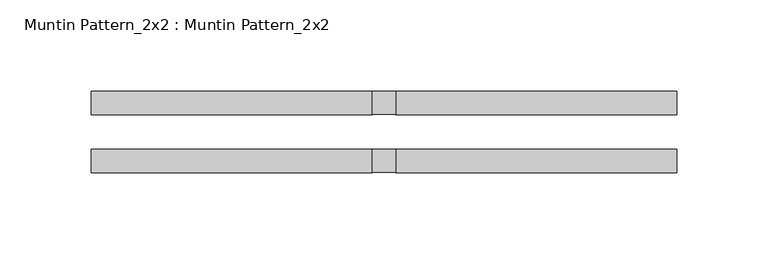
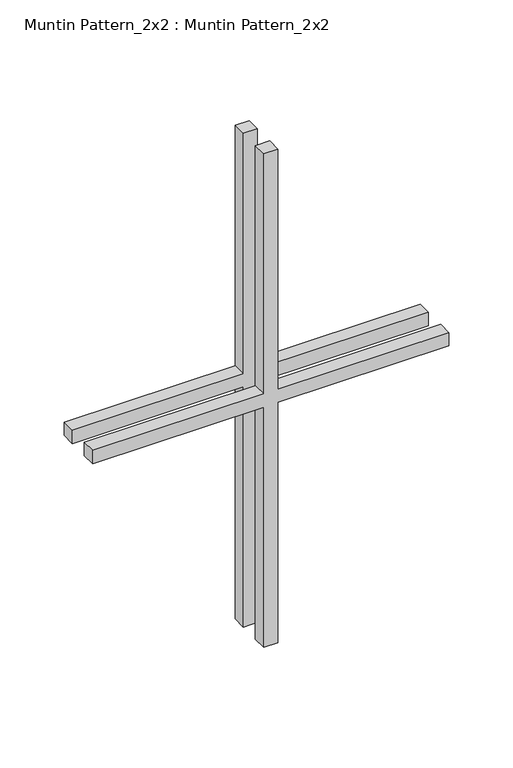
"""IFC4 building model written with IfcOpenShell, lengths in millimetres: proxy geometry, Muntin Pattern_2x2 : Muntin Pattern_2x2."""

from ifc_helpers import new_model, si_unit, frame, origin, place, context, project, spatial, polyline, outline, extrude, source, transform, mapped, element, save


def muntin_pattern_2x2_muntin_pattern_2x2_27d56209(model_context):
    return source(origin(), model_context, "Body", "SweptSolid", [
        extrude(outline(polyline([(241.3, -6.35), (241.3, -160.3375), (228.6, -160.3375), (228.6, -6.35), (0.0, -6.35), (0.0, 6.35), (228.6, 6.35), (228.6, 160.3375), (241.3, 160.3375), (241.3, 6.35), (469.9, 6.35), (469.9, -6.35), (241.3, -6.35)])), frame((0.0, 9.525, 0.0), z_axis=(0.0, 1.0, 0.0), x_axis=(0.0, 0.0, 1.0)), (0.0, 0.0, 1.0), 12.7),
        extrude(outline(polyline([(241.3, -6.35), (241.3, -160.3375), (228.6, -160.3375), (228.6, -6.35), (0.0, -6.35), (0.0, 6.35), (228.6, 6.35), (228.6, 160.3375), (241.3, 160.3375), (241.3, 6.35), (469.9, 6.35), (469.9, -6.35), (241.3, -6.35)])), frame((0.0, -22.225, 0.0), z_axis=(0.0, 1.0, 0.0), x_axis=(0.0, 0.0, 1.0)), (0.0, 0.0, 1.0), 12.7),
    ])


if __name__ == "__main__":
    model = new_model("IFC4")
    model_context = context("Model", 3, world=origin())
    ifc_project = project(units=[si_unit("LENGTHUNIT", "METRE", prefix="MILLI")], contexts=[model_context])
    site = spatial("IfcSite", under=ifc_project)
    building = spatial("IfcBuilding", under=site)
    placement = place(None, origin())
    muntin_pattern_2x2_muntin_pattern_2x2_shape = muntin_pattern_2x2_muntin_pattern_2x2_27d56209(model_context)
    element("IfcBuildingElementProxy", 1, Name="Muntin Pattern_2x2 : Muntin Pattern_2x2", ObjectType="Muntin Pattern_2x2 : Muntin Pattern_2x2", at=placement, inside=building, context=model_context, shape_type="MappedRepresentation", body=[
        mapped(muntin_pattern_2x2_muntin_pattern_2x2_shape, transform((0.0, 0.0, 0.0), x_axis=(1.0, 0.0, 0.0), y_axis=(0.0, 1.0, 0.0), z_axis=(0.0, 0.0, 1.0))),
    ])
    save(model, "model.ifc")

# Revit data of these elements
# Type "Muntin Pattern_2x2 : Muntin Pattern_2x2"
#   Width [instance default] = 48"
#   Thickness = 0.5"
#   Height [instance default] = 48"
#   Distance = 0.75"
#   Interior Material [instance default] = none
#   Exterior Material [instance default] = none
#   Default Elevation = 0
# Element 1 (IfcBuildingElementProxy, "Muntin Pattern_2x2 : Muntin Pattern_2x2")
#   Width = 12.625"
#   Height = 18.5"
#   Interior Material = Wood - Stained
#   Exterior Material = Clad - White
#   Materials on its faces: "Clad - White", "Wood - Stained"
# Materials
#   "Clad - White": class "Wood", colour RGB 242 242 238, transparency 0, Cost = 0
#   "Wood - Stained": class "Wood", colour RGB 224 178 126, transparency 0, Cost = 0
